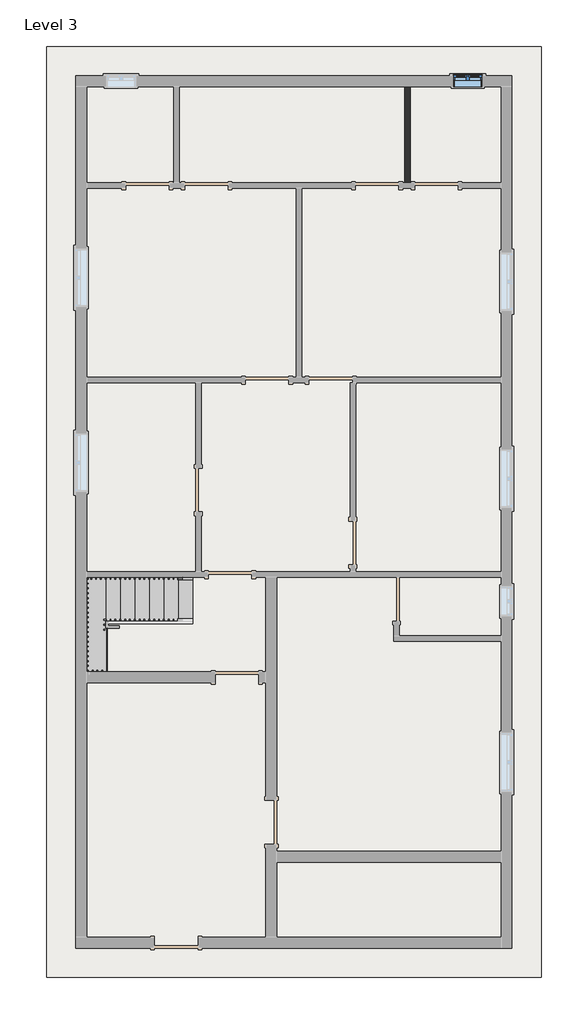
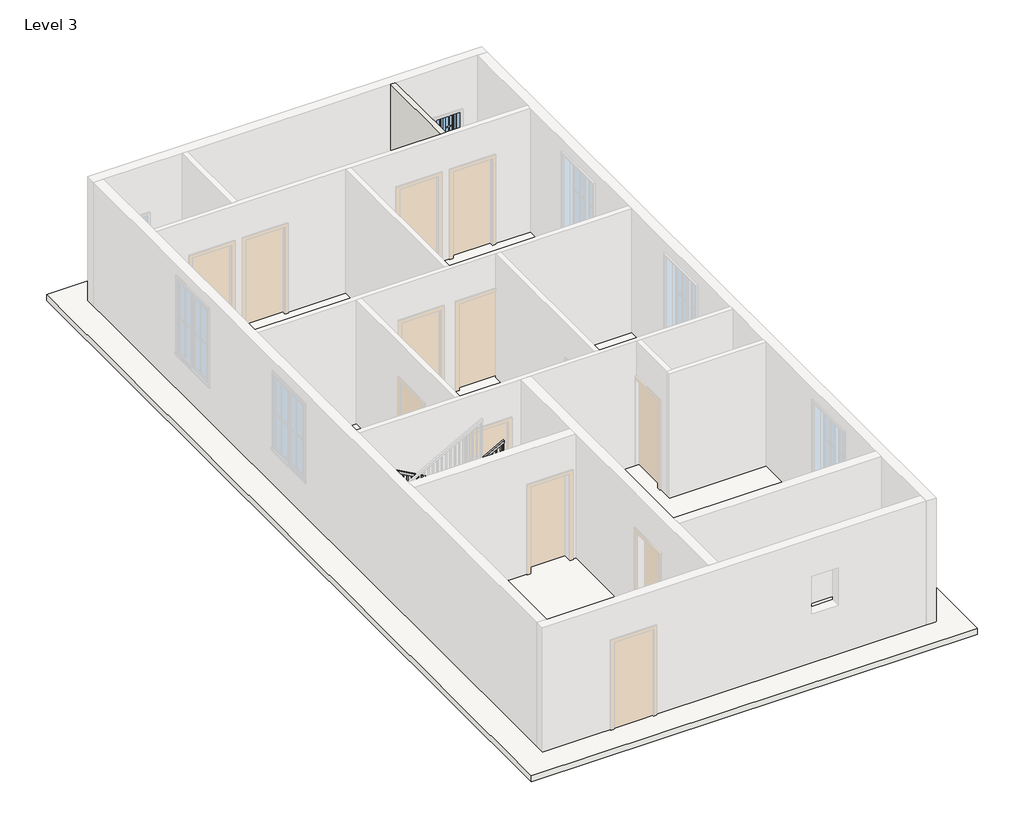
# One storey, part 2 of 3: 1 railing, 1 slab, 1 stair flight, 1 wall, 1 window.
"""IFC4 building model written with IfcOpenShell, lengths in millimetres."""

from ifc_helpers import new_model, si_unit, frame, origin, place, context, project, spatial, polyline, outline, extrude, faceted_brep, transform, mapped, element, save
from components import stair_flight_cd429425, window_c417fced

model = new_model("IFC4")

# Units and contexts
model_context = context("Model", 3, world=origin())
ifc_project = project(units=[si_unit("LENGTHUNIT", "METRE", prefix="MILLI")], contexts=[model_context])

# Site, building, storey
site = spatial("IfcSite", under=ifc_project)
building = spatial("IfcBuilding", under=site)
storey = spatial("IfcBuildingStorey", under=building, Name="Level 3", Elevation=6096.0)

# Railing
placement = place(None, origin())
element("IfcRailing", 1, ObjectType="Handrail - Rectangular", at=placement, inside=storey, context=model_context, shape_type="SolidModel", body=[
    faceted_brep([(3727.9146873, 3657.6, 7179.7333333), (3727.9146873, 3657.6, 7121.620221), (3727.9146873, 3708.4, 7121.620221), (3727.9146873, 3708.4, 7179.7333333), (1899.1146873, 3657.6, 8195.7333333), (1885.9510851, 3657.6, 8144.9333333), (1885.9510851, 3708.4, 8144.9333333), (1899.1146873, 3708.4, 8195.7333333), (1549.4, 3657.6, 8195.7333333), (1549.4, 3657.6, 8144.9333333), (1498.6, 3708.4, 8144.9333333), (1498.6, 3708.4, 8195.7333333), (1549.4, 1778.0, 8195.7333333), (1549.4, 1778.0, 8144.9333333), (1498.6, 1727.2, 8144.9333333), (1498.6, 1727.2, 8195.7333333), (1594.3146873, 1778.0, 8195.7333333), (1607.4782895, 1778.0, 8144.9333333), (1607.4782895, 1727.2, 8144.9333333), (1594.3146873, 1727.2, 8195.7333333), (3727.9146873, 1778.0, 9381.0666667), (3727.9146873, 1727.2, 9381.0666667), (3727.9146873, 1727.2, 9322.9535543), (3727.9146873, 1778.0, 9322.9535543)], [[[0, 1, 2, 3]], [[1, 0, 4, 5]], [[2, 1, 5, 6]], [[3, 2, 6, 7]], [[0, 3, 7, 4]], [[5, 4, 8, 9]], [[6, 5, 9, 10]], [[7, 6, 10, 11]], [[4, 7, 11, 8]], [[9, 8, 12, 13]], [[10, 9, 13, 14]], [[11, 10, 14, 15]], [[8, 11, 15, 12]], [[13, 12, 16, 17]], [[14, 13, 17, 18]], [[15, 14, 18, 19]], [[12, 15, 19, 16]], [[20, 21, 22, 23]], [[17, 16, 20, 23]], [[18, 17, 23, 22]], [[19, 18, 22, 21]], [[16, 19, 21, 20]]]),
    extrude(outline(polyline([(9289.1815058, 3667.125), (9278.5981725, 3648.075), (8297.3333333, 3648.075), (8297.3333333, 3667.125), (9289.1815058, 3667.125)])), frame((0.0, 1743.075, 0.0), z_axis=(0.0, 1.0, 0.0), x_axis=(0.0, 0.0, 1.0)), (0.0, 0.0, 1.0), 19.05),
    extrude(outline(polyline([(9232.7370614, 3565.525), (9222.153728, 3546.475), (8297.3333333, 3546.475), (8297.3333333, 3565.525), (9232.7370614, 3565.525)])), frame((0.0, 1743.075, 0.0), z_axis=(0.0, 1.0, 0.0), x_axis=(0.0, 0.0, 1.0)), (0.0, 0.0, 1.0), 19.05),
    extrude(outline(polyline([(9176.2926169, 3463.925), (9165.7092836, 3444.875), (8297.3333333, 3444.875), (8297.3333333, 3463.925), (9176.2926169, 3463.925)])), frame((0.0, 1743.075, 0.0), z_axis=(0.0, 1.0, 0.0), x_axis=(0.0, 0.0, 1.0)), (0.0, 0.0, 1.0), 19.05),
    extrude(outline(polyline([(9119.8481725, 3362.325), (9109.2648391, 3343.275), (8128.0, 3343.275), (8128.0, 3362.325), (9119.8481725, 3362.325)])), frame((0.0, 1743.075, 0.0), z_axis=(0.0, 1.0, 0.0), x_axis=(0.0, 0.0, 1.0)), (0.0, 0.0, 1.0), 19.05),
    extrude(outline(polyline([(9063.403728, 3260.725), (9052.8203947, 3241.675), (8128.0, 3241.675), (8128.0, 3260.725), (9063.403728, 3260.725)])), frame((0.0, 1743.075, 0.0), z_axis=(0.0, 1.0, 0.0), x_axis=(0.0, 0.0, 1.0)), (0.0, 0.0, 1.0), 19.05),
    extrude(outline(polyline([(9006.9592836, 3159.125), (8996.3759503, 3140.075), (8128.0, 3140.075), (8128.0, 3159.125), (9006.9592836, 3159.125)])), frame((0.0, 1743.075, 0.0), z_axis=(0.0, 1.0, 0.0), x_axis=(0.0, 0.0, 1.0)), (0.0, 0.0, 1.0), 19.05),
    extrude(outline(polyline([(8950.5148391, 3057.525), (8939.9315058, 3038.475), (7958.6666667, 3038.475), (7958.6666667, 3057.525), (8950.5148391, 3057.525)])), frame((0.0, 1743.075, 0.0), z_axis=(0.0, 1.0, 0.0), x_axis=(0.0, 0.0, 1.0)), (0.0, 0.0, 1.0), 19.05),
    extrude(outline(polyline([(8894.0703947, 2955.925), (8883.4870614, 2936.875), (7958.6666667, 2936.875), (7958.6666667, 2955.925), (8894.0703947, 2955.925)])), frame((0.0, 1743.075, 0.0), z_axis=(0.0, 1.0, 0.0), x_axis=(0.0, 0.0, 1.0)), (0.0, 0.0, 1.0), 19.05),
    extrude(outline(polyline([(8837.6259503, 2854.325), (8827.0426169, 2835.275), (7958.6666667, 2835.275), (7958.6666667, 2854.325), (8837.6259503, 2854.325)])), frame((0.0, 1743.075, 0.0), z_axis=(0.0, 1.0, 0.0), x_axis=(0.0, 0.0, 1.0)), (0.0, 0.0, 1.0), 19.05),
    extrude(outline(polyline([(8781.1815058, 2752.725), (8770.5981725, 2733.675), (7789.3333333, 2733.675), (7789.3333333, 2752.725), (8781.1815058, 2752.725)])), frame((0.0, 1743.075, 0.0), z_axis=(0.0, 1.0, 0.0), x_axis=(0.0, 0.0, 1.0)), (0.0, 0.0, 1.0), 19.05),
    extrude(outline(polyline([(8724.7370614, 2651.125), (8714.153728, 2632.075), (7789.3333333, 2632.075), (7789.3333333, 2651.125), (8724.7370614, 2651.125)])), frame((0.0, 1743.075, 0.0), z_axis=(0.0, 1.0, 0.0), x_axis=(0.0, 0.0, 1.0)), (0.0, 0.0, 1.0), 19.05),
    extrude(outline(polyline([(8668.2926169, 2549.525), (8657.7092836, 2530.475), (7789.3333333, 2530.475), (7789.3333333, 2549.525), (8668.2926169, 2549.525)])), frame((0.0, 1743.075, 0.0), z_axis=(0.0, 1.0, 0.0), x_axis=(0.0, 0.0, 1.0)), (0.0, 0.0, 1.0), 19.05),
    extrude(outline(polyline([(8611.8481725, 2447.925), (8601.2648391, 2428.875), (7620.0, 2428.875), (7620.0, 2447.925), (8611.8481725, 2447.925)])), frame((0.0, 1743.075, 0.0), z_axis=(0.0, 1.0, 0.0), x_axis=(0.0, 0.0, 1.0)), (0.0, 0.0, 1.0), 19.05),
    extrude(outline(polyline([(8555.403728, 2346.325), (8544.8203947, 2327.275), (7620.0, 2327.275), (7620.0, 2346.325), (8555.403728, 2346.325)])), frame((0.0, 1743.075, 0.0), z_axis=(0.0, 1.0, 0.0), x_axis=(0.0, 0.0, 1.0)), (0.0, 0.0, 1.0), 19.05),
    extrude(outline(polyline([(8498.9592836, 2244.725), (8488.3759503, 2225.675), (7620.0, 2225.675), (7620.0, 2244.725), (8498.9592836, 2244.725)])), frame((0.0, 1743.075, 0.0), z_axis=(0.0, 1.0, 0.0), x_axis=(0.0, 0.0, 1.0)), (0.0, 0.0, 1.0), 19.05),
    extrude(outline(polyline([(8442.5148391, 2143.125), (8431.9315058, 2124.075), (7450.6666667, 2124.075), (7450.6666667, 2143.125), (8442.5148391, 2143.125)])), frame((0.0, 1743.075, 0.0), z_axis=(0.0, 1.0, 0.0), x_axis=(0.0, 0.0, 1.0)), (0.0, 0.0, 1.0), 19.05),
    extrude(outline(polyline([(8386.0703947, 2041.525), (8375.4870614, 2022.475), (7450.6666667, 2022.475), (7450.6666667, 2041.525), (8386.0703947, 2041.525)])), frame((0.0, 1743.075, 0.0), z_axis=(0.0, 1.0, 0.0), x_axis=(0.0, 0.0, 1.0)), (0.0, 0.0, 1.0), 19.05),
    extrude(outline(polyline([(8329.6259503, 1939.925), (8319.0426169, 1920.875), (7450.6666667, 1920.875), (7450.6666667, 1939.925), (8329.6259503, 1939.925)])), frame((0.0, 1743.075, 0.0), z_axis=(0.0, 1.0, 0.0), x_axis=(0.0, 0.0, 1.0)), (0.0, 0.0, 1.0), 19.05),
    extrude(outline(polyline([(8273.1815058, 1838.325), (8262.5981725, 1819.275), (7281.3333333, 1819.275), (7281.3333333, 1838.325), (8273.1815058, 1838.325)])), frame((0.0, 1743.075, 0.0), z_axis=(0.0, 1.0, 0.0), x_axis=(0.0, 0.0, 1.0)), (0.0, 0.0, 1.0), 19.05),
    extrude(outline(polyline([(8216.7370614, 1736.725), (8206.153728, 1717.675), (7281.3333333, 1717.675), (7281.3333333, 1736.725), (8216.7370614, 1736.725)])), frame((0.0, 1743.075, 0.0), z_axis=(0.0, 1.0, 0.0), x_axis=(0.0, 0.0, 1.0)), (0.0, 0.0, 1.0), 19.05),
    extrude(outline(polyline([(8160.2926169, 1635.125), (8149.7092836, 1616.075), (7281.3333333, 1616.075), (7281.3333333, 1635.125), (8160.2926169, 1635.125)])), frame((0.0, 1743.075, 0.0), z_axis=(0.0, 1.0, 0.0), x_axis=(0.0, 0.0, 1.0)), (0.0, 0.0, 1.0), 19.05),
    extrude(outline(polyline([(1514.475, 1863.725), (1533.525, 1863.725), (1533.525, 1844.675), (1514.475, 1844.675), (1514.475, 1863.725)])), frame((0.0, 0.0, 7281.3333333), z_axis=(0.0, 0.0, 1.0), x_axis=(1.0, 0.0, 0.0)), (0.0, 0.0, 1.0), 863.6),
    extrude(outline(polyline([(1514.475, 1965.325), (1533.525, 1965.325), (1533.525, 1946.275), (1514.475, 1946.275), (1514.475, 1965.325)])), frame((0.0, 0.0, 7281.3333333), z_axis=(0.0, 0.0, 1.0), x_axis=(1.0, 0.0, 0.0)), (0.0, 0.0, 1.0), 863.6),
    extrude(outline(polyline([(1514.475, 2066.925), (1533.525, 2066.925), (1533.525, 2047.875), (1514.475, 2047.875), (1514.475, 2066.925)])), frame((0.0, 0.0, 7281.3333333), z_axis=(0.0, 0.0, 1.0), x_axis=(1.0, 0.0, 0.0)), (0.0, 0.0, 1.0), 863.6),
    extrude(outline(polyline([(1514.475, 2168.525), (1533.525, 2168.525), (1533.525, 2149.475), (1514.475, 2149.475), (1514.475, 2168.525)])), frame((0.0, 0.0, 7281.3333333), z_axis=(0.0, 0.0, 1.0), x_axis=(1.0, 0.0, 0.0)), (0.0, 0.0, 1.0), 863.6),
    extrude(outline(polyline([(1514.475, 2270.125), (1533.525, 2270.125), (1533.525, 2251.075), (1514.475, 2251.075), (1514.475, 2270.125)])), frame((0.0, 0.0, 7281.3333333), z_axis=(0.0, 0.0, 1.0), x_axis=(1.0, 0.0, 0.0)), (0.0, 0.0, 1.0), 863.6),
    extrude(outline(polyline([(1514.475, 2371.725), (1533.525, 2371.725), (1533.525, 2352.675), (1514.475, 2352.675), (1514.475, 2371.725)])), frame((0.0, 0.0, 7281.3333333), z_axis=(0.0, 0.0, 1.0), x_axis=(1.0, 0.0, 0.0)), (0.0, 0.0, 1.0), 863.6),
    extrude(outline(polyline([(1514.475, 2473.325), (1533.525, 2473.325), (1533.525, 2454.275), (1514.475, 2454.275), (1514.475, 2473.325)])), frame((0.0, 0.0, 7281.3333333), z_axis=(0.0, 0.0, 1.0), x_axis=(1.0, 0.0, 0.0)), (0.0, 0.0, 1.0), 863.6),
    extrude(outline(polyline([(1514.475, 2574.925), (1533.525, 2574.925), (1533.525, 2555.875), (1514.475, 2555.875), (1514.475, 2574.925)])), frame((0.0, 0.0, 7281.3333333), z_axis=(0.0, 0.0, 1.0), x_axis=(1.0, 0.0, 0.0)), (0.0, 0.0, 1.0), 863.6),
    extrude(outline(polyline([(1514.475, 2676.525), (1533.525, 2676.525), (1533.525, 2657.475), (1514.475, 2657.475), (1514.475, 2676.525)])), frame((0.0, 0.0, 7281.3333333), z_axis=(0.0, 0.0, 1.0), x_axis=(1.0, 0.0, 0.0)), (0.0, 0.0, 1.0), 863.6),
    extrude(outline(polyline([(1514.475, 2778.125), (1533.525, 2778.125), (1533.525, 2759.075), (1514.475, 2759.075), (1514.475, 2778.125)])), frame((0.0, 0.0, 7281.3333333), z_axis=(0.0, 0.0, 1.0), x_axis=(1.0, 0.0, 0.0)), (0.0, 0.0, 1.0), 863.6),
    extrude(outline(polyline([(1514.475, 2879.725), (1533.525, 2879.725), (1533.525, 2860.675), (1514.475, 2860.675), (1514.475, 2879.725)])), frame((0.0, 0.0, 7281.3333333), z_axis=(0.0, 0.0, 1.0), x_axis=(1.0, 0.0, 0.0)), (0.0, 0.0, 1.0), 863.6),
    extrude(outline(polyline([(1514.475, 2981.325), (1533.525, 2981.325), (1533.525, 2962.275), (1514.475, 2962.275), (1514.475, 2981.325)])), frame((0.0, 0.0, 7281.3333333), z_axis=(0.0, 0.0, 1.0), x_axis=(1.0, 0.0, 0.0)), (0.0, 0.0, 1.0), 863.6),
    extrude(outline(polyline([(1514.475, 3082.925), (1533.525, 3082.925), (1533.525, 3063.875), (1514.475, 3063.875), (1514.475, 3082.925)])), frame((0.0, 0.0, 7281.3333333), z_axis=(0.0, 0.0, 1.0), x_axis=(1.0, 0.0, 0.0)), (0.0, 0.0, 1.0), 863.6),
    extrude(outline(polyline([(1514.475, 3184.525), (1533.525, 3184.525), (1533.525, 3165.475), (1514.475, 3165.475), (1514.475, 3184.525)])), frame((0.0, 0.0, 7281.3333333), z_axis=(0.0, 0.0, 1.0), x_axis=(1.0, 0.0, 0.0)), (0.0, 0.0, 1.0), 863.6),
    extrude(outline(polyline([(1514.475, 3286.125), (1533.525, 3286.125), (1533.525, 3267.075), (1514.475, 3267.075), (1514.475, 3286.125)])), frame((0.0, 0.0, 7281.3333333), z_axis=(0.0, 0.0, 1.0), x_axis=(1.0, 0.0, 0.0)), (0.0, 0.0, 1.0), 863.6),
    extrude(outline(polyline([(1514.475, 3387.725), (1533.525, 3387.725), (1533.525, 3368.675), (1514.475, 3368.675), (1514.475, 3387.725)])), frame((0.0, 0.0, 7281.3333333), z_axis=(0.0, 0.0, 1.0), x_axis=(1.0, 0.0, 0.0)), (0.0, 0.0, 1.0), 863.6),
    extrude(outline(polyline([(1514.475, 3489.325), (1533.525, 3489.325), (1533.525, 3470.275), (1514.475, 3470.275), (1514.475, 3489.325)])), frame((0.0, 0.0, 7281.3333333), z_axis=(0.0, 0.0, 1.0), x_axis=(1.0, 0.0, 0.0)), (0.0, 0.0, 1.0), 863.6),
    extrude(outline(polyline([(1514.475, 3590.925), (1533.525, 3590.925), (1533.525, 3571.875), (1514.475, 3571.875), (1514.475, 3590.925)])), frame((0.0, 0.0, 7281.3333333), z_axis=(0.0, 0.0, 1.0), x_axis=(1.0, 0.0, 0.0)), (0.0, 0.0, 1.0), 863.6),
    extrude(outline(polyline([(1603.8396873, 3692.525), (1603.8396873, 3673.475), (1584.7896873, 3673.475), (1584.7896873, 3692.525), (1603.8396873, 3692.525)])), frame((0.0, 0.0, 7281.3333333), z_axis=(0.0, 0.0, 1.0), x_axis=(1.0, 0.0, 0.0)), (0.0, 0.0, 1.0), 863.6),
    extrude(outline(polyline([(1705.4396873, 3692.525), (1705.4396873, 3673.475), (1686.3896873, 3673.475), (1686.3896873, 3692.525), (1705.4396873, 3692.525)])), frame((0.0, 0.0, 7281.3333333), z_axis=(0.0, 0.0, 1.0), x_axis=(1.0, 0.0, 0.0)), (0.0, 0.0, 1.0), 863.6),
    extrude(outline(polyline([(1807.0396873, 3692.525), (1807.0396873, 3673.475), (1787.9896873, 3673.475), (1787.9896873, 3692.525), (1807.0396873, 3692.525)])), frame((0.0, 0.0, 7281.3333333), z_axis=(0.0, 0.0, 1.0), x_axis=(1.0, 0.0, 0.0)), (0.0, 0.0, 1.0), 863.6),
    extrude(outline(polyline([(8132.3285543, 1908.6396873), (8142.9118876, 1889.5896873), (7281.3333333, 1889.5896873), (7281.3333333, 1908.6396873), (8132.3285543, 1908.6396873)])), frame((0.0, 3673.475, 0.0), z_axis=(0.0, 1.0, 0.0), x_axis=(0.0, 0.0, 1.0)), (0.0, 0.0, 1.0), 19.05),
    extrude(outline(polyline([(8075.8841099, 2010.2396873), (8086.4674432, 1991.1896873), (7112.0, 1991.1896873), (7112.0, 2010.2396873), (8075.8841099, 2010.2396873)])), frame((0.0, 3673.475, 0.0), z_axis=(0.0, 1.0, 0.0), x_axis=(0.0, 0.0, 1.0)), (0.0, 0.0, 1.0), 19.05),
    extrude(outline(polyline([(8019.4396654, 2111.8396873), (8030.0229988, 2092.7896873), (7112.0, 2092.7896873), (7112.0, 2111.8396873), (8019.4396654, 2111.8396873)])), frame((0.0, 3673.475, 0.0), z_axis=(0.0, 1.0, 0.0), x_axis=(0.0, 0.0, 1.0)), (0.0, 0.0, 1.0), 19.05),
    extrude(outline(polyline([(7962.995221, 2213.4396873), (7973.5785543, 2194.3896873), (7112.0, 2194.3896873), (7112.0, 2213.4396873), (7962.995221, 2213.4396873)])), frame((0.0, 3673.475, 0.0), z_axis=(0.0, 1.0, 0.0), x_axis=(0.0, 0.0, 1.0)), (0.0, 0.0, 1.0), 19.05),
    extrude(outline(polyline([(7906.5507765, 2315.0396873), (7917.1341099, 2295.9896873), (6942.6666667, 2295.9896873), (6942.6666667, 2315.0396873), (7906.5507765, 2315.0396873)])), frame((0.0, 3673.475, 0.0), z_axis=(0.0, 1.0, 0.0), x_axis=(0.0, 0.0, 1.0)), (0.0, 0.0, 1.0), 19.05),
    extrude(outline(polyline([(7850.1063321, 2416.6396873), (7860.6896654, 2397.5896873), (6942.6666667, 2397.5896873), (6942.6666667, 2416.6396873), (7850.1063321, 2416.6396873)])), frame((0.0, 3673.475, 0.0), z_axis=(0.0, 1.0, 0.0), x_axis=(0.0, 0.0, 1.0)), (0.0, 0.0, 1.0), 19.05),
    extrude(outline(polyline([(7793.6618876, 2518.2396873), (7804.245221, 2499.1896873), (6942.6666667, 2499.1896873), (6942.6666667, 2518.2396873), (7793.6618876, 2518.2396873)])), frame((0.0, 3673.475, 0.0), z_axis=(0.0, 1.0, 0.0), x_axis=(0.0, 0.0, 1.0)), (0.0, 0.0, 1.0), 19.05),
    extrude(outline(polyline([(7737.2174432, 2619.8396873), (7747.8007765, 2600.7896873), (6773.3333333, 2600.7896873), (6773.3333333, 2619.8396873), (7737.2174432, 2619.8396873)])), frame((0.0, 3673.475, 0.0), z_axis=(0.0, 1.0, 0.0), x_axis=(0.0, 0.0, 1.0)), (0.0, 0.0, 1.0), 19.05),
    extrude(outline(polyline([(7680.7729988, 2721.4396873), (7691.3563321, 2702.3896873), (6773.3333333, 2702.3896873), (6773.3333333, 2721.4396873), (7680.7729988, 2721.4396873)])), frame((0.0, 3673.475, 0.0), z_axis=(0.0, 1.0, 0.0), x_axis=(0.0, 0.0, 1.0)), (0.0, 0.0, 1.0), 19.05),
    extrude(outline(polyline([(7624.3285543, 2823.0396873), (7634.9118876, 2803.9896873), (6773.3333333, 2803.9896873), (6773.3333333, 2823.0396873), (7624.3285543, 2823.0396873)])), frame((0.0, 3673.475, 0.0), z_axis=(0.0, 1.0, 0.0), x_axis=(0.0, 0.0, 1.0)), (0.0, 0.0, 1.0), 19.05),
    extrude(outline(polyline([(7567.8841099, 2924.6396873), (7578.4674432, 2905.5896873), (6604.0, 2905.5896873), (6604.0, 2924.6396873), (7567.8841099, 2924.6396873)])), frame((0.0, 3673.475, 0.0), z_axis=(0.0, 1.0, 0.0), x_axis=(0.0, 0.0, 1.0)), (0.0, 0.0, 1.0), 19.05),
    extrude(outline(polyline([(7511.4396654, 3026.2396873), (7522.0229988, 3007.1896873), (6604.0, 3007.1896873), (6604.0, 3026.2396873), (7511.4396654, 3026.2396873)])), frame((0.0, 3673.475, 0.0), z_axis=(0.0, 1.0, 0.0), x_axis=(0.0, 0.0, 1.0)), (0.0, 0.0, 1.0), 19.05),
    extrude(outline(polyline([(7454.995221, 3127.8396873), (7465.5785543, 3108.7896873), (6604.0, 3108.7896873), (6604.0, 3127.8396873), (7454.995221, 3127.8396873)])), frame((0.0, 3673.475, 0.0), z_axis=(0.0, 1.0, 0.0), x_axis=(0.0, 0.0, 1.0)), (0.0, 0.0, 1.0), 19.05),
    extrude(outline(polyline([(7398.5507765, 3229.4396873), (7409.1341099, 3210.3896873), (6434.6666667, 3210.3896873), (6434.6666667, 3229.4396873), (7398.5507765, 3229.4396873)])), frame((0.0, 3673.475, 0.0), z_axis=(0.0, 1.0, 0.0), x_axis=(0.0, 0.0, 1.0)), (0.0, 0.0, 1.0), 19.05),
    extrude(outline(polyline([(7342.1063321, 3331.0396873), (7352.6896654, 3311.9896873), (6434.6666667, 3311.9896873), (6434.6666667, 3331.0396873), (7342.1063321, 3331.0396873)])), frame((0.0, 3673.475, 0.0), z_axis=(0.0, 1.0, 0.0), x_axis=(0.0, 0.0, 1.0)), (0.0, 0.0, 1.0), 19.05),
    extrude(outline(polyline([(7285.6618876, 3432.6396873), (7296.245221, 3413.5896873), (6434.6666667, 3413.5896873), (6434.6666667, 3432.6396873), (7285.6618876, 3432.6396873)])), frame((0.0, 3673.475, 0.0), z_axis=(0.0, 1.0, 0.0), x_axis=(0.0, 0.0, 1.0)), (0.0, 0.0, 1.0), 19.05),
    extrude(outline(polyline([(7229.2174432, 3534.2396873), (7239.8007765, 3515.1896873), (6265.3333333, 3515.1896873), (6265.3333333, 3534.2396873), (7229.2174432, 3534.2396873)])), frame((0.0, 3673.475, 0.0), z_axis=(0.0, 1.0, 0.0), x_axis=(0.0, 0.0, 1.0)), (0.0, 0.0, 1.0), 19.05),
    extrude(outline(polyline([(7172.7729988, 3635.8396873), (7183.3563321, 3616.7896873), (6265.3333333, 3616.7896873), (6265.3333333, 3635.8396873), (7172.7729988, 3635.8396873)])), frame((0.0, 3673.475, 0.0), z_axis=(0.0, 1.0, 0.0), x_axis=(0.0, 0.0, 1.0)), (0.0, 0.0, 1.0), 19.05),
    extrude(outline(polyline([(1514.475, 1762.125), (1533.525, 1762.125), (1533.525, 1743.075), (1514.475, 1743.075), (1514.475, 1762.125)])), frame((0.0, 0.0, 7281.3333333), z_axis=(0.0, 0.0, 1.0), x_axis=(1.0, 0.0, 0.0)), (0.0, 0.0, 1.0), 863.6),
    extrude(outline(polyline([(1533.525, 3692.525), (1533.525, 3673.475), (1514.475, 3673.475), (1514.475, 3692.525), (1533.525, 3692.525)])), frame((0.0, 0.0, 7281.3333333), z_axis=(0.0, 0.0, 1.0), x_axis=(1.0, 0.0, 0.0)), (0.0, 0.0, 1.0), 863.6),
    extrude(outline(polyline([(9322.9535543, 3727.9146873), (9312.370221, 3708.8646873), (8297.3333333, 3708.8646873), (8297.3333333, 3727.9146873), (9322.9535543, 3727.9146873)])), frame((0.0, 1743.075, 0.0), z_axis=(0.0, 1.0, 0.0), x_axis=(0.0, 0.0, 1.0)), (0.0, 0.0, 1.0), 19.05),
    extrude(outline(polyline([(7121.620221, 3727.9146873), (7132.2035543, 3708.8646873), (6265.3333333, 3708.8646873), (6265.3333333, 3727.9146873), (7121.620221, 3727.9146873)])), frame((0.0, 3673.475, 0.0), z_axis=(0.0, 1.0, 0.0), x_axis=(0.0, 0.0, 1.0)), (0.0, 0.0, 1.0), 19.05),
])

# Slab
element("IfcSlab", 2, ObjectType="Generic - 12\"", at=placement, inside=storey, context=model_context, shape_type="SweptSolid", body=[
    extrude(outline(polyline([(11023.6, 14833.6), (11023.6, -4673.6), (660.4, -4673.6), (660.4, 14833.6), (11023.6, 14833.6)])), frame((0.0, 0.0, 5943.6), z_axis=(0.0, 0.0, 1.0), x_axis=(1.0, 0.0, 0.0)), (0.0, 0.0, 1.0), 152.4),
])

# Stair flight
stair_flight_shape = stair_flight_cd429425(model_context)
element("IfcStairFlight", 3, ObjectType="2\" Tread 1\" Nosing 1/4\" Riser", at=placement, inside=storey, context=model_context, shape_type="MappedRepresentation", body=[
    mapped(stair_flight_shape, transform((0.0, 0.0, 0.0), x_axis=(1.0, 0.0, 0.0), y_axis=(0.0, 1.0, 0.0), z_axis=(0.0, 0.0, 1.0))),
])

# Wall
element("IfcWall", 4, ObjectType="Generic - 5\"", at=placement, inside=storey, context=model_context, shape_type="SweptSolid", body=[
    extrude(outline(polyline([(8166.1, 11976.1), (8166.1, 13995.4), (8280.4, 13995.4), (8280.4, 11976.1), (8166.1, 11976.1)])), frame((0.0, 0.0, 6096.0), z_axis=(0.0, 0.0, 1.0), x_axis=(1.0, 0.0, 0.0)), (0.0, 0.0, 1.0), 3048.0),
])

# Window
window_shape = window_c417fced(model_context)
element("IfcWindow", 5, ObjectType="Window-Casement-Double : 24\" x 36\"", at=placement, inside=storey, context=model_context, shape_type="MappedRepresentation", body=[
    mapped(window_shape, transform((9486.9, 14109.7, 6096.0), x_axis=(1.0, 0.0, 0.0), y_axis=(0.0, 1.0, 0.0), z_axis=(0.0, 0.0, 1.0))),
])

save(model, "model.ifc")

# Revit data of these elements
# Type "Handrail - Rectangular"
#   Assembly Code = "C2010400"
#   built-in parameter 1008612 = 0.0416667 (stored number, unit not read)
#   built-in parameter 1008611 = 0.0416667 (stored number, unit not read)
#   built-in parameter 1008609 = 0.333333 (stored number, unit not read)
#   built-in parameter 1008604 = 0.166667 (stored number, unit not read)
#   built-in parameter 1008603 = 0.166667 (stored number, unit not read)
#   Railing Height = 3' - 0"
#   built-in parameter 1008630 = 2
#   built-in parameter 1008610 = 2
#   built-in parameter 1008618 = Baluster - Square : 3/4"
# Type "Generic - 12\""
#   Assembly Code = "B1010"
#   Function = 0
#   Layers, outside or top first: 0' - 6" "Door - Panel" (function 1)
# Type "Generic - 5\""
#   Assembly Code = "B2010"
#   Layers, outside or top first: 0' - 4 1/2" no material (function 1)
# Type "Window-Casement-Double : 24\" x 36\""
#   Type Mark = "14"
#   Fire Rating = "0.5h"
#   Assembly Code = "B2020100"
#   Analytic Construction = "Double glazing - domestic"
#   Frame Extension [instance default] = 0' - 0 1/4"
#   Window Inset [instance default] = 0' - 0"
#   Wall Thickness [instance default] = 0' - 6"
#   Interior Wall Closure [instance default] = 0' - 2 1/4"
#   Half Width = 1' - 0"
#   Visual Light Transmittance = 0.81
#   Thermal Resistance (R) = 1.8146 (h·ft²·°F)/BTU
#   Solar Heat Gain Coefficient = 0.76
#   Rough Width = 2' - 0 1/2"
#   Rough Height = 3' - 0 1/2"
#   Height = 3' - 0"
#   Heat Transfer Coefficient (U) = 0.5511 BTU/(h·ft²·°F)
#   Exterior Wall Closure [instance default] = 0' - 1 1/4"
#   Extension Jamb [instance default] = 0' - 2 1/4"
#   Default Sill Height = 3' - 0"
#   Width = 2' - 0"
#   Define Thermal Properties by = 0
#   Muntin Visibility = yes
#   Interior Trim Visibility [instance default] = yes
#   Exterior Trim Visibility [instance default] = yes
#   Extension Jamb Visibility [instance default] = yes
#   Interior Trim Material = Wood - Stained
#   Muntin Pattern = Muntin Pattern_2x2 : Muntin Pattern_2x2
#   Interior Trim = Trim-Window-Interior-Flat : Picture Frame
#   Interior Frame Material = Wood - Stained
#   Glass Panel Material = Glass
#   Exterior Trim Material = Clad - White
#   Exterior Trim = Trim-Window-Exterior-Flat : with Sill
#   Exterior Frame Material = Clad - White
#   Wall Closure = (empty or 0)
# Element 1 (IfcRailing, "Handrail - Rectangular")
#   Phase Created = New Construction
# Element 2 (IfcSlab, "Generic - 12\"")
#   Height Offset From Level = 0' - 0"
#   Phase Created = New Construction
#   Materials on its faces: "Door - Panel"
# Element 3 (IfcStairFlight, "2\" Tread 1\" Nosing 1/4\" Riser")
#   Phase Created = New Construction
# Element 4 (IfcWall, "Generic - 5\"")
#   Top Offset = 0' - 0"
#   Base Offset = 0' - 0"
#   wall height = 10' - 0"
#   Phase Created = New Construction
#   Base Constraint = Level 3
#   Top Constraint = Level 4
#   Materials on its faces: "Default Wall"
# Element 5 (IfcWindow, "Window-Casement-Double : 24\" x 36\"")
#   Mark = "23"
#   Window Inset = 0' - 0"
#   Interior Wall Closure = 0' - 2 1/4"
#   Frame Extension = 0' - 0 1/4"
#   Exterior Wall Closure = 0' - 1 1/4"
#   Interior Trim Visibility = yes
#   Exterior Trim Visibility = yes
#   Phase Created = New Construction
#   Materials on its faces: "Wood - Stained", "Glass", "Clad - White"
# Materials
#   "Door - Panel": class "Wood", colour RGB 210 159 95, transparency 0, Cost = 0
#   "Wood - Stained": class "Wood", colour RGB 224 178 126, transparency 0, Cost = 0
#   "Glass": class "Glass", colour RGB 0 128 192, transparency 0.75, Description = "Soda Lime Glass", Cost = 0
#   "Clad - White": class "Wood", colour RGB 242 242 238, transparency 0, Cost = 0
#   "Default Wall": colour RGB 128 128 128, transparency 0, Cost = 0
